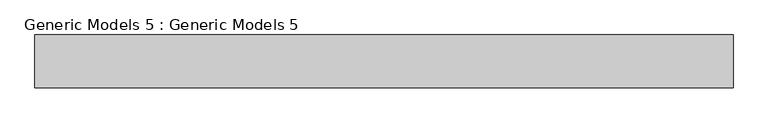
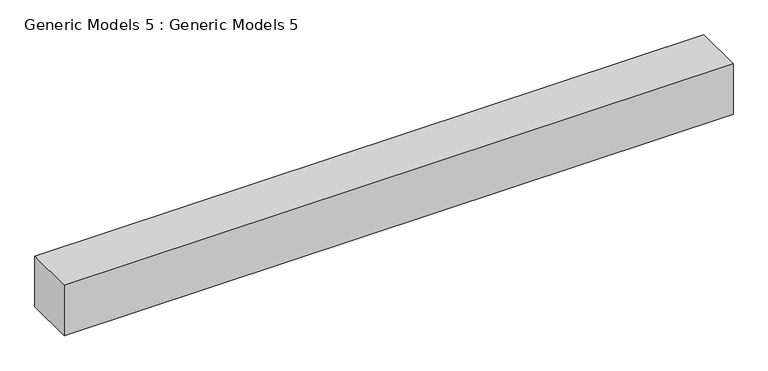
"""IFC4 building model written with IfcOpenShell, lengths in millimetres: proxy geometry, Generic Models 5 : Generic Models 5."""

from ifc_helpers import new_model, si_unit, frame, origin, place, context, project, spatial, polyline, outline, extrude, source, transform, mapped, element, save


def generic_models_5_generic_models_5_43fa52cd(model_context):
    return source(origin(), model_context, "Body", "SweptSolid", [
        extrude(outline(polyline([(4030.4306032, -8681.0497532), (4030.4306032, -9747.8497532), (-10060.7625896, -9747.8497532), (-10060.7625896, -8681.0497532), (4030.4306032, -8681.0497532)])), frame((0.0, 0.0, 11081.1477648), z_axis=(0.0, 0.0, 1.0), x_axis=(1.0, 0.0, 0.0)), (0.0, 0.0, 1.0), 1123.7332522),
    ])


if __name__ == "__main__":
    model = new_model("IFC4")
    model_context = context("Model", 3, world=origin())
    ifc_project = project(units=[si_unit("LENGTHUNIT", "METRE", prefix="MILLI")], contexts=[model_context])
    site = spatial("IfcSite", under=ifc_project)
    building = spatial("IfcBuilding", under=site)
    placement = place(None, origin())
    generic_models_5_generic_models_5_shape = generic_models_5_generic_models_5_43fa52cd(model_context)
    element("IfcBuildingElementProxy", 1, Name="Generic Models 5 : Generic Models 5", ObjectType="Generic Models 5 : Generic Models 5", at=placement, inside=building, context=model_context, shape_type="MappedRepresentation", body=[
        mapped(generic_models_5_generic_models_5_shape, transform((0.0, 0.0, 0.0), x_axis=(1.0, 0.0, 0.0), y_axis=(0.0, 1.0, 0.0), z_axis=(0.0, 0.0, 1.0))),
    ])
    save(model, "model.ifc")
